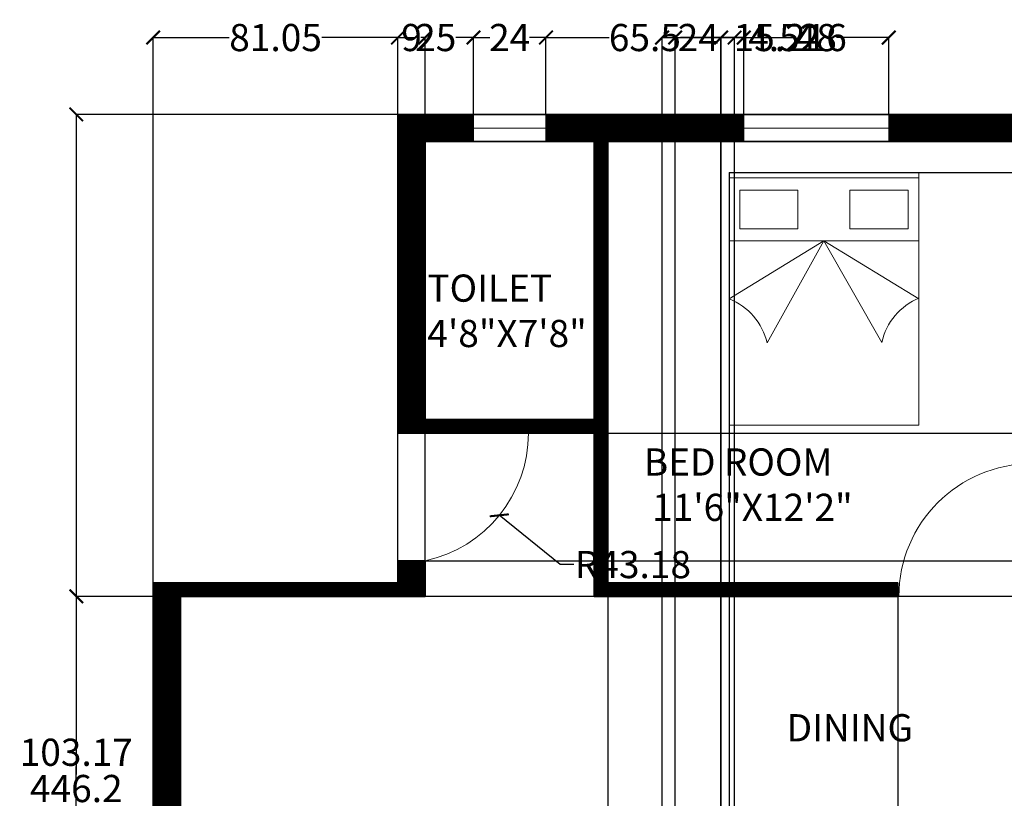
# Model space of a CAD drawing. Units: inches. Extents: x -43 to 552, y 22 to 537.
# Tile 2 of 4: x -43 to 283, y 280 to 537. Entities that reach past the tile are written whole.
import ezdxf

# ---------------------------------------------------------------- set-up
doc = ezdxf.new("R2010")
doc.units = ezdxf.units.IN
doc.header["$MEASUREMENT"] = 0
for name, color, linetype, lineweight in [('A-ANNO-DIMS', 2, 'Continuous', 18), ('A-AREA-IDEN', 7, 'Continuous', 18), ('A-DOOR', 4, 'Continuous', 18), ('A-FURN', 8, 'Continuous', 18), ('A-GLAZ', 4, 'Continuous', 18), ('A-WALL', 7, 'Continuous', 35), ('A-WALL-PATT', 252, 'Continuous', 13)]:
    doc.layers.add(name, color=color, linetype=linetype, lineweight=lineweight)
doc.styles.get("Standard").update_dxf_attribs({"font": 'arial.ttf'})
doc.dimstyles.get("Standard").update_dxf_attribs({"dimtxt": 9, "dimasz": 4.5, "dimexe": 0.18, "dimexo": 0.0625, "dimgap": 0.09, "dimtad": 0, "dimtih": 1, "dimtoh": 1, "dimdec": 1, "dimzin": 0, "dimdsep": 46, "dimlunit": 4, "dimtxsty": 'Standard', "dimblk": 'ARCHTICK', "dimcen": 0.09, "dimadec": 0, "dimazin": 0, "dimtfac": 1, "dimtdec": 1, "dimtofl": 0, "dimtmove": 0, "dimatfit": 3, "dimfxl": 1, "dimtolj": 1, "dimtzin": 0, "dimarcsym": 0})

# ---------------------------------------------------------------- blocks, each defined once
blk = doc.blocks.new('BED-DOUBLE')
for p, q in [((0, 83.65), (62.74, 83.65)), ((0, 0), (0, 83.65)), ((0, 81.91), (62.74, 81.91)), ((62.74, 83.65), (62.74, 0)), ((0, 61), (62.74, 61)), ((31.37, 61), (0, 41.83)), ((12.53, 27.23), (31.37, 61)), ((62.74, 41.83), (31.37, 61)), ((31.37, 61), (50.51, 27.4)), ((62.74, 0), (0, 0))]:
    blk.add_line(p, q)
for points in [[(3.55, 77.79), (22.76, 77.79), (22.76, 64.95), (3.55, 64.95)], [(59.19, 77.79), (39.98, 77.79), (39.98, 64.95), (59.19, 64.95)]]:
    blk.add_lwpolyline(points, close=True)
for centre, start, end in [((-7.65, 22.59), 12.9482, 68.3142), ((70.73, 22.94), 112.1918, 167.5578)]:
    blk.add_arc(centre, 20.7, start, end)
blk = doc.blocks.new('_ArchTick')
at = {"color": 0, "linetype": 'ByBlock', "const_width": 0.15}
blk.add_lwpolyline([(-0.5, -0.5), (0.5, 0.5)], dxfattribs=at)
blk = doc.blocks.new('*D9')
at = {"layer": 'A-ANNO-DIMS', "color": 0, "lineweight": -2, "transparency": 16777216}
for p, q in [((82.45, 505.95), (-24.17, 505.95)), ((-23.99, 505.95), (-23.99, 287.55)), ((-23.99, 59.77), (-23.99, 278.18)), ((289.95, 59.77), (-24.17, 59.77))]:
    blk.add_line(p, q, dxfattribs=at)
at = {"layer": 'Defpoints', "color": 0, "transparency": 16777216}
for p in [(-23.99, 505.95), (82.51, 505.95), (290.01, 59.77)]:
    blk.add_point(p, dxfattribs=at)
at = {"layer": 'A-ANNO-DIMS', "color": 0, "lineweight": -2, "transparency": 16777216, "xscale": 4.5, "yscale": 4.5, "zscale": 4.5}
for p, rotation in [((-23.99, 505.95), 90), ((-23.99, 59.77), 270)]:
    blk.add_blockref('_ArchTick', p, dxfattribs=dict(at, rotation=rotation))
at = {"layer": 'A-ANNO-DIMS', "color": 0, "transparency": 16777216, "insert": (-23.99, 282.86), "char_height": 9, "attachment_point": 5}
blk.add_mtext('\\A1;446.2', dxfattribs=at)
blk = doc.blocks.new('*D10')
at = {"layer": 'A-ANNO-DIMS', "color": 0, "lineweight": -2, "transparency": 16777216}
for p, q in [((1.46, 351.01), (1.46, 531.58)), ((1.46, 531.4), (26.67, 531.4)), ((82.51, 531.4), (57.3, 531.4)), ((82.51, 506.01), (82.51, 531.58))]:
    blk.add_line(p, q, dxfattribs=at)
at = {"layer": 'Defpoints', "color": 0, "transparency": 16777216}
for p in [(82.51, 531.4), (82.51, 505.95), (1.46, 350.95)]:
    blk.add_point(p, dxfattribs=at)
at = {"layer": 'A-ANNO-DIMS', "color": 0, "lineweight": -2, "transparency": 16777216, "xscale": 4.5, "yscale": 4.5, "zscale": 4.5, "rotation": 180}
blk.add_blockref('_ArchTick', (1.46, 531.4), dxfattribs=at)
at = {"layer": 'A-ANNO-DIMS', "color": 0, "lineweight": -2, "transparency": 16777216, "xscale": 4.5, "yscale": 4.5, "zscale": 4.5}
blk.add_blockref('_ArchTick', (82.51, 531.4), dxfattribs=at)
at = {"layer": 'A-ANNO-DIMS', "color": 0, "transparency": 16777216, "insert": (41.99, 531.4), "char_height": 9, "attachment_point": 5}
blk.add_mtext('\\A1;81.05', dxfattribs=at)
blk = doc.blocks.new('*D11')
at = {"layer": 'A-ANNO-DIMS', "color": 0, "lineweight": -2, "transparency": 16777216}
for p, q in [((82.51, 506.01), (82.51, 531.58)), ((82.51, 531.4), (88.36, 531.4)), ((107.51, 531.4), (101.66, 531.4)), ((107.51, 506.01), (107.51, 531.58))]:
    blk.add_line(p, q, dxfattribs=at)
at = {"layer": 'Defpoints', "color": 0, "transparency": 16777216}
for p in [(107.51, 531.4), (82.51, 505.95), (107.51, 505.95)]:
    blk.add_point(p, dxfattribs=at)
at = {"layer": 'A-ANNO-DIMS', "color": 0, "lineweight": -2, "transparency": 16777216, "xscale": 4.5, "yscale": 4.5, "zscale": 4.5, "rotation": 180}
blk.add_blockref('_ArchTick', (82.51, 531.4), dxfattribs=at)
at = {"layer": 'A-ANNO-DIMS', "color": 0, "lineweight": -2, "transparency": 16777216, "xscale": 4.5, "yscale": 4.5, "zscale": 4.5}
blk.add_blockref('_ArchTick', (107.51, 531.4), dxfattribs=at)
at = {"layer": 'A-ANNO-DIMS', "color": 0, "transparency": 16777216, "insert": (95.01, 531.4), "char_height": 9, "attachment_point": 5}
blk.add_mtext('\\A1;25', dxfattribs=at)
blk = doc.blocks.new('*D12')
at = {"layer": 'A-ANNO-DIMS', "color": 0, "lineweight": -2, "transparency": 16777216}
for p, q in [((107.51, 506.01), (107.51, 531.58)), ((107.51, 531.4), (112.92, 531.4)), ((131.51, 531.4), (126.11, 531.4)), ((131.51, 506.01), (131.51, 531.58))]:
    blk.add_line(p, q, dxfattribs=at)
at = {"layer": 'Defpoints', "color": 0, "transparency": 16777216}
for p in [(131.51, 531.4), (107.51, 505.95), (131.51, 505.95)]:
    blk.add_point(p, dxfattribs=at)
at = {"layer": 'A-ANNO-DIMS', "color": 0, "lineweight": -2, "transparency": 16777216, "xscale": 4.5, "yscale": 4.5, "zscale": 4.5, "rotation": 180}
blk.add_blockref('_ArchTick', (107.51, 531.4), dxfattribs=at)
at = {"layer": 'A-ANNO-DIMS', "color": 0, "lineweight": -2, "transparency": 16777216, "xscale": 4.5, "yscale": 4.5, "zscale": 4.5}
blk.add_blockref('_ArchTick', (131.51, 531.4), dxfattribs=at)
at = {"layer": 'A-ANNO-DIMS', "color": 0, "transparency": 16777216, "insert": (119.51, 531.4), "char_height": 9, "attachment_point": 5}
blk.add_mtext('\\A1;24', dxfattribs=at)
blk = doc.blocks.new('*D13')
at = {"layer": 'A-ANNO-DIMS', "color": 0, "lineweight": -2, "transparency": 16777216}
for p, q in [((131.51, 506.01), (131.51, 531.58)), ((131.51, 531.4), (152.42, 531.4)), ((197.01, 531.4), (176.1, 531.4)), ((197.01, 506.01), (197.01, 531.58))]:
    blk.add_line(p, q, dxfattribs=at)
at = {"layer": 'Defpoints', "color": 0, "transparency": 16777216}
for p in [(197.01, 531.4), (131.51, 505.95), (197.01, 505.95)]:
    blk.add_point(p, dxfattribs=at)
at = {"layer": 'A-ANNO-DIMS', "color": 0, "lineweight": -2, "transparency": 16777216, "xscale": 4.5, "yscale": 4.5, "zscale": 4.5, "rotation": 180}
blk.add_blockref('_ArchTick', (131.51, 531.4), dxfattribs=at)
at = {"layer": 'A-ANNO-DIMS', "color": 0, "lineweight": -2, "transparency": 16777216, "xscale": 4.5, "yscale": 4.5, "zscale": 4.5}
blk.add_blockref('_ArchTick', (197.01, 531.4), dxfattribs=at)
at = {"layer": 'A-ANNO-DIMS', "color": 0, "transparency": 16777216, "insert": (164.26, 531.4), "char_height": 9, "attachment_point": 5}
blk.add_mtext('\\A1;65.5', dxfattribs=at)
blk = doc.blocks.new('*D14')
at = {"layer": 'A-ANNO-DIMS', "color": 0, "lineweight": -2, "transparency": 16777216}
for p, q in [((197.01, 506.01), (197.01, 531.58)), ((197.01, 531.4), (214.28, 531.4)), ((245.01, 531.4), (227.74, 531.4)), ((245.01, 506.01), (245.01, 531.58))]:
    blk.add_line(p, q, dxfattribs=at)
at = {"layer": 'Defpoints', "color": 0, "transparency": 16777216}
for p in [(245.01, 531.4), (197.01, 505.95), (245.01, 505.95)]:
    blk.add_point(p, dxfattribs=at)
at = {"layer": 'A-ANNO-DIMS', "color": 0, "lineweight": -2, "transparency": 16777216, "xscale": 4.5, "yscale": 4.5, "zscale": 4.5, "rotation": 180}
blk.add_blockref('_ArchTick', (197.01, 531.4), dxfattribs=at)
at = {"layer": 'A-ANNO-DIMS', "color": 0, "lineweight": -2, "transparency": 16777216, "xscale": 4.5, "yscale": 4.5, "zscale": 4.5}
blk.add_blockref('_ArchTick', (245.01, 531.4), dxfattribs=at)
at = {"layer": 'A-ANNO-DIMS', "color": 0, "transparency": 16777216, "insert": (221.01, 531.4), "char_height": 9, "attachment_point": 5}
blk.add_mtext('\\A1;48', dxfattribs=at)
blk = doc.blocks.new('*D29')
at = {"layer": 'A-ANNO-DIMS', "color": 0, "lineweight": -2, "transparency": 16777216}
for p, q in [((364.95, 346.45), (-24.17, 346.45)), ((-23.99, 346.45), (-23.99, 299.55)), ((-23.99, 243.27), (-23.99, 290.17)), ((364.95, 243.27), (-24.17, 243.27))]:
    blk.add_line(p, q, dxfattribs=at)
at = {"layer": 'Defpoints', "color": 0, "transparency": 16777216}
for p in [(-23.99, 346.45), (365.01, 346.45), (365.01, 243.27)]:
    blk.add_point(p, dxfattribs=at)
at = {"layer": 'A-ANNO-DIMS', "color": 0, "lineweight": -2, "transparency": 16777216, "xscale": 4.5, "yscale": 4.5, "zscale": 4.5}
for p, rotation in [((-23.99, 346.45), 90), ((-23.99, 243.27), 270)]:
    blk.add_blockref('_ArchTick', p, dxfattribs=dict(at, rotation=rotation))
at = {"layer": 'A-ANNO-DIMS', "color": 0, "transparency": 16777216, "insert": (-23.99, 294.86), "char_height": 9, "attachment_point": 5}
blk.add_mtext('\\A1;103.17', dxfattribs=at)
blk = doc.blocks.new('*D31')
at = {"layer": 'A-ANNO-DIMS', "color": 0, "lineweight": -2, "transparency": 16777216}
for p, q in [((82.51, 358.28), (82.51, 531.58)), ((82.51, 531.4), (83.96, 531.4)), ((91.51, 531.4), (90.06, 531.4)), ((91.51, 358.28), (91.51, 531.58))]:
    blk.add_line(p, q, dxfattribs=at)
at = {"layer": 'Defpoints', "color": 0, "transparency": 16777216}
for p in [(91.51, 531.4), (82.51, 358.22), (91.51, 358.22)]:
    blk.add_point(p, dxfattribs=at)
at = {"layer": 'A-ANNO-DIMS', "color": 0, "lineweight": -2, "transparency": 16777216, "xscale": 4.5, "yscale": 4.5, "zscale": 4.5, "rotation": 180}
blk.add_blockref('_ArchTick', (82.51, 531.4), dxfattribs=at)
at = {"layer": 'A-ANNO-DIMS', "color": 0, "lineweight": -2, "transparency": 16777216, "xscale": 4.5, "yscale": 4.5, "zscale": 4.5}
blk.add_blockref('_ArchTick', (91.51, 531.4), dxfattribs=at)
at = {"layer": 'A-ANNO-DIMS', "color": 0, "transparency": 16777216, "insert": (87.01, 531.4), "char_height": 9, "attachment_point": 5}
blk.add_mtext('\\A1;9', dxfattribs=at)
blk = doc.blocks.new('*D36')
at = {"layer": 'A-ANNO-DIMS', "color": 0, "lineweight": -2, "transparency": 16777216}
for p, q in [((82.57, 400.45), (533.19, 400.45)), ((533.01, 400.45), (533.01, 384.02)), ((533.01, 358.22), (533.01, 374.64)), ((82.57, 358.22), (533.19, 358.22))]:
    blk.add_line(p, q, dxfattribs=at)
at = {"layer": 'Defpoints', "color": 0, "transparency": 16777216}
for p in [(82.51, 400.45), (533.01, 400.45), (82.51, 358.22)]:
    blk.add_point(p, dxfattribs=at)
at = {"layer": 'A-ANNO-DIMS', "color": 0, "lineweight": -2, "transparency": 16777216, "xscale": 4.5, "yscale": 4.5, "zscale": 4.5}
for p, rotation in [((533.01, 400.45), 90), ((533.01, 358.22), 270)]:
    blk.add_blockref('_ArchTick', p, dxfattribs=dict(at, rotation=rotation))
at = {"layer": 'A-ANNO-DIMS', "color": 0, "transparency": 16777216, "insert": (533.01, 379.33), "char_height": 9, "attachment_point": 5}
blk.add_mtext('\\A1;42.23', dxfattribs=at)
blk = doc.blocks.new('*D37')
at = {"layer": 'A-ANNO-DIMS', "color": 0, "lineweight": -2, "transparency": 16777216}
for p, q in [((248.01, 346.38), (248.01, 34.14)), ((290.01, 346.38), (290.01, 34.14)), ((248.01, 34.32), (262.34, 34.32)), ((290.01, 34.32), (275.68, 34.32))]:
    blk.add_line(p, q, dxfattribs=at)
at = {"layer": 'Defpoints', "color": 0, "transparency": 16777216}
for p in [(248.01, 346.45), (290.01, 346.45), (290.01, 34.32)]:
    blk.add_point(p, dxfattribs=at)
at = {"layer": 'A-ANNO-DIMS', "color": 0, "lineweight": -2, "transparency": 16777216, "xscale": 4.5, "yscale": 4.5, "zscale": 4.5, "rotation": 180}
blk.add_blockref('_ArchTick', (248.01, 34.32), dxfattribs=at)
at = {"layer": 'A-ANNO-DIMS', "color": 0, "lineweight": -2, "transparency": 16777216, "xscale": 4.5, "yscale": 4.5, "zscale": 4.5}
blk.add_blockref('_ArchTick', (290.01, 34.32), dxfattribs=at)
at = {"layer": 'A-ANNO-DIMS', "color": 0, "transparency": 16777216, "insert": (269.01, 34.32), "char_height": 9, "attachment_point": 5}
blk.add_mtext('\\A1;42', dxfattribs=at)
blk = doc.blocks.new('*D39')
at = {"layer": 'A-ANNO-DIMS', "color": 0, "lineweight": -2, "transparency": 16777216}
for p, q in [((152.01, 496.88), (152.01, 34.14)), ((192.19, 486.68), (192.19, 34.14)), ((152.01, 34.32), (156.63, 34.32)), ((192.19, 34.32), (187.56, 34.32))]:
    blk.add_line(p, q, dxfattribs=at)
at = {"layer": 'Defpoints', "color": 0, "transparency": 16777216}
for p in [(152.01, 496.95), (192.19, 486.74), (192.19, 34.32)]:
    blk.add_point(p, dxfattribs=at)
at = {"layer": 'A-ANNO-DIMS', "color": 0, "lineweight": -2, "transparency": 16777216, "xscale": 4.5, "yscale": 4.5, "zscale": 4.5, "rotation": 180}
blk.add_blockref('_ArchTick', (152.01, 34.32), dxfattribs=at)
at = {"layer": 'A-ANNO-DIMS', "color": 0, "lineweight": -2, "transparency": 16777216, "xscale": 4.5, "yscale": 4.5, "zscale": 4.5}
blk.add_blockref('_ArchTick', (192.19, 34.32), dxfattribs=at)
at = {"layer": 'A-ANNO-DIMS', "color": 0, "transparency": 16777216, "insert": (172.1, 34.32), "char_height": 9, "attachment_point": 5}
blk.add_mtext('\\A1;40.18', dxfattribs=at)
blk = doc.blocks.new('*D40')
at = {"layer": 'A-ANNO-DIMS', "color": 0, "lineweight": -2, "transparency": 16777216}
for p, q in [((197.07, 496.95), (533.19, 496.95)), ((533.01, 496.95), (533.01, 496.53)), ((192.25, 486.74), (533.19, 486.74)), ((533.01, 486.74), (533.01, 487.16))]:
    blk.add_line(p, q, dxfattribs=at)
at = {"layer": 'Defpoints', "color": 0, "transparency": 16777216}
for p in [(197.01, 496.95), (533.01, 496.95), (192.19, 486.74)]:
    blk.add_point(p, dxfattribs=at)
at = {"layer": 'A-ANNO-DIMS', "color": 0, "lineweight": -2, "transparency": 16777216, "xscale": 4.5, "yscale": 4.5, "zscale": 4.5}
for p, rotation in [((533.01, 496.95), 90), ((533.01, 486.74), 270)]:
    blk.add_blockref('_ArchTick', p, dxfattribs=dict(at, rotation=rotation))
at = {"layer": 'A-ANNO-DIMS', "color": 0, "transparency": 16777216, "insert": (533.01, 491.84), "char_height": 9, "attachment_point": 5}
blk.add_mtext('\\A1;10.204', dxfattribs=at)
blk = doc.blocks.new('*D44')
at = {"layer": 'A-ANNO-DIMS', "color": 0, "lineweight": -2, "transparency": 16777216}
for p, q in [((169.96, 255.18), (169.96, 531.58)), ((169.96, 531.4), (175.37, 531.4)), ((193.96, 531.4), (188.56, 531.4)), ((193.96, 255.18), (193.96, 531.58))]:
    blk.add_line(p, q, dxfattribs=at)
at = {"layer": 'Defpoints', "color": 0, "transparency": 16777216}
for p in [(193.96, 531.4), (169.96, 255.12), (193.96, 255.12)]:
    blk.add_point(p, dxfattribs=at)
at = {"layer": 'A-ANNO-DIMS', "color": 0, "lineweight": -2, "transparency": 16777216, "xscale": 4.5, "yscale": 4.5, "zscale": 4.5, "rotation": 180}
blk.add_blockref('_ArchTick', (169.96, 531.4), dxfattribs=at)
at = {"layer": 'A-ANNO-DIMS', "color": 0, "lineweight": -2, "transparency": 16777216, "xscale": 4.5, "yscale": 4.5, "zscale": 4.5}
blk.add_blockref('_ArchTick', (193.96, 531.4), dxfattribs=at)
at = {"layer": 'A-ANNO-DIMS', "color": 0, "transparency": 16777216, "insert": (181.96, 531.4), "char_height": 9, "attachment_point": 5}
blk.add_mtext('\\A1;24', dxfattribs=at)
blk = doc.blocks.new('*D49')
at = {"layer": 'A-ANNO-DIMS', "color": 0, "lineweight": -2, "transparency": 16777216}
for p, q in [((174.31, 245.11), (174.31, 531.58)), ((174.31, 531.4), (189.53, 531.4)), ((189.53, 245.11), (189.53, 531.58)), ((189.53, 531.4), (194.03, 531.4))]:
    blk.add_line(p, q, dxfattribs=at)
at = {"layer": 'Defpoints', "color": 0, "transparency": 16777216}
for p in [(189.53, 531.4), (174.31, 245.05), (189.53, 245.05)]:
    blk.add_point(p, dxfattribs=at)
at = {"layer": 'A-ANNO-DIMS', "color": 0, "lineweight": -2, "transparency": 16777216, "xscale": 4.5, "yscale": 4.5, "zscale": 4.5, "rotation": 180}
blk.add_blockref('_ArchTick', (174.31, 531.4), dxfattribs=at)
at = {"layer": 'A-ANNO-DIMS', "color": 0, "lineweight": -2, "transparency": 16777216, "xscale": 4.5, "yscale": 4.5, "zscale": 4.5}
blk.add_blockref('_ArchTick', (189.53, 531.4), dxfattribs=at)
at = {"layer": 'A-ANNO-DIMS', "color": 0, "transparency": 16777216, "insert": (212.37, 531.4), "char_height": 9, "attachment_point": 5}
blk.add_mtext('\\A1;15.216', dxfattribs=at)
blk = doc.blocks.new('*D53')
at = {"layer": 'A-ANNO-DIMS', "color": 0, "lineweight": -2, "transparency": 16777216}
for p, q in [((189.45, 165.34), (189.45, 531.58)), ((189.45, 531.4), (193.96, 531.4)), ((193.96, 146.51), (193.96, 531.58)), ((193.96, 531.4), (198.46, 531.4))]:
    blk.add_line(p, q, dxfattribs=at)
at = {"layer": 'Defpoints', "color": 0, "transparency": 16777216}
for p in [(193.96, 531.4), (189.45, 165.27), (193.96, 146.45)]:
    blk.add_point(p, dxfattribs=at)
at = {"layer": 'A-ANNO-DIMS', "color": 0, "lineweight": -2, "transparency": 16777216, "xscale": 4.5, "yscale": 4.5, "zscale": 4.5, "rotation": 180}
blk.add_blockref('_ArchTick', (189.45, 531.4), dxfattribs=at)
at = {"layer": 'A-ANNO-DIMS', "color": 0, "lineweight": -2, "transparency": 16777216, "xscale": 4.5, "yscale": 4.5, "zscale": 4.5}
blk.add_blockref('_ArchTick', (193.96, 531.4), dxfattribs=at)
at = {"layer": 'A-ANNO-DIMS', "color": 0, "transparency": 16777216, "insert": (210.38, 531.4), "char_height": 9, "attachment_point": 5}
blk.add_mtext('\\A1;4.52', dxfattribs=at)
blk = doc.blocks.new('*D56')
at = {"layer": 'A-ANNO-DIMS', "color": 0, "lineweight": -2, "transparency": 16777216}
for p, q in [((82.42, 400.45), (82.6, 400.45)), ((82.51, 400.36), (82.51, 400.54)), ((136.21, 356.98), (116.07, 373.28)), ((140.71, 356.98), (136.21, 356.98))]:
    blk.add_line(p, q, dxfattribs=at)
at = {"layer": 'Defpoints', "color": 0, "transparency": 16777216}
for p in [(82.51, 400.45), (116.07, 373.28)]:
    blk.add_point(p, dxfattribs=at)
at = {"layer": 'A-ANNO-DIMS', "color": 0, "lineweight": -2, "transparency": 16777216, "xscale": 4.5, "yscale": 4.5, "zscale": 4.5, "rotation": 141.0154171181597}
blk.add_blockref('_ArchTick', (116.07, 373.28), dxfattribs=at)
at = {"layer": 'A-ANNO-DIMS', "color": 0, "transparency": 16777216, "insert": (160.3, 356.98), "char_height": 9, "attachment_point": 5}
blk.add_mtext('\\A1;R43.18', dxfattribs=at)

msp = doc.modelspace()

# ---------------------------------------------------------------- hatches: boundary and pattern name
at = {"layer": 'A-WALL-PATT'}
h = msp.add_hatch(dxfattribs=at)
h.set_pattern_fill('ANSI31', color=256)
h.set_pattern_definition([(45, (-523.11303, 0), (-0.088388348, 0.088388348), [])])
h.paths.add_polyline_path([(202.9985, 146.4471), (169.965, 146.4471), (169.965, 255.1157), (165.465, 255.1157), (165.465, 146.4471), (147.9805, 146.4471), (147.9805, 141.9471), (165.465, 141.9471), (165.465, 84.9471), (169.965, 84.9471), (169.965, 141.9471), (202.9985, 141.9471)])
h.paths.add_polyline_path([(294.5106, 146.4471), (294.5106, 238.775), (294.5106, 243.275), (294.5106, 255.1157), (290.0106, 255.1157), (290.0106, 146.4471), (247.8411, 146.4471), (247.8411, 141.9471), (290.0106, 141.9471), (290.0106, 93.9471), (290.0106, 59.775), (294.5106, 59.775), (294.5106, 77.3814), (294.5106, 93.9471), (294.5106, 107.775), (316.2676, 107.775), (316.2676, 116.775), (294.5106, 116.775)])
h.paths.add_polyline_path([(10.465, 346.4471), (82.5106, 346.4471), (91.5106, 346.4471), (91.5106, 358.2163), (82.5106, 358.2163), (82.5106, 350.9471), (1.465, 350.9471), (1.465, 84.9471), (10.465, 84.9471), (10.465, 141.9471), (56.4237, 141.9471), (56.4237, 146.4471), (10.465, 146.4471)])
h.paths.add_polyline_path([(91.5106, 496.9471), (107.5106, 496.9471), (107.5106, 505.9471), (82.5106, 505.9471), (82.5106, 400.4471), (147.5106, 400.4471), (147.5106, 346.4471), (248.0106, 346.4471), (248.0106, 350.9471), (152.0106, 350.9471), (152.0106, 496.9471), (197.0106, 496.9471), (197.0106, 505.9471), (131.5106, 505.9471), (131.5106, 496.9471), (147.5106, 496.9471), (147.5106, 404.9471), (91.5106, 404.9471)])
h.paths.add_polyline_path([(477.5106, 505.9471), (245.0106, 505.9471), (245.0106, 496.9471), (290.0106, 496.9471), (290.0106, 390.2693, -0.02565505), (294.5106, 390.2693), (294.5106, 496.9471), (468.5106, 496.9471), (468.5106, 460.1763), (477.5106, 460.1763)])

# ---------------------------------------------------------------- linework, layer by layer
at = {"layer": 'A-DOOR'}
for p, q in [((82.5106, 400.4471), (82.5106, 358.2163)), ((290.0106, 346.4471), (248.0106, 346.4471)), ((248.0106, 346.4471), (294.5106, 346.4471))]:
    msp.add_line(p, q, dxfattribs=at)
for centre, radius, start, end in [((82.5106, 400.4471), 43.1792, 282.030572, 0), ((292.2606, 346.4471), 43.8799, 0, 180)]:
    msp.add_arc(centre, radius, start, end, dxfattribs=at)
at = {"layer": 'A-GLAZ'}
for p, q in [((107.5106, 496.9471), (107.5106, 505.9471)), ((131.5106, 496.9471), (131.5106, 505.9471)), ((197.0106, 496.9471), (197.0106, 505.9471)), ((245.0106, 496.9471), (245.0106, 505.9471)), ((107.5106, 501.4471), (131.5106, 501.4471)), ((197.0106, 501.4471), (245.0106, 501.4471))]:
    msp.add_line(p, q, dxfattribs=at)
at = {"layer": 'A-WALL'}
for p, q in [((82.5106, 505.9471), (477.5106, 505.9471)), ((82.5106, 505.9471), (82.5106, 400.4471)), ((91.5106, 496.9471), (147.5106, 496.9471)), ((91.5106, 496.9471), (91.5106, 404.9471)), ((147.5106, 496.9471), (147.5106, 404.9471)), ((152.0106, 496.9471), (152.0106, 350.9471)), ((152.0106, 496.9471), (290.0106, 496.9471)), ((91.5106, 404.9471), (147.5106, 404.9471)), ((82.5106, 400.4471), (147.5106, 400.4471)), ((147.5106, 400.4471), (147.5106, 346.4471)), ((82.5106, 358.2163), (91.5106, 358.2163)), ((82.5106, 358.2163), (82.5106, 350.9471)), ((91.5106, 358.2163), (91.5106, 346.4471)), ((1.465, 350.9471), (1.465, 84.9471)), ((82.5106, 350.9471), (1.465, 350.9471)), ((152.0106, 350.9471), (248.0106, 350.9471)), ((248.0106, 350.9471), (248.0106, 346.4471)), ((10.465, 346.4471), (10.465, 146.4471)), ((82.5106, 346.4471), (10.465, 346.4471)), ((82.5106, 346.4471), (91.5106, 346.4471)), ((147.5106, 346.4471), (248.0106, 346.4471))]:
    msp.add_line(p, q, dxfattribs=at)

# ---------------------------------------------------------------- block references
at = {"layer": 'A-FURN'}
msp.add_blockref('BED-DOUBLE', (192.1876, 403.0902), dxfattribs=at)

# ---------------------------------------------------------------- texts
at = {"layer": 'A-AREA-IDEN', "char_height": 9, "attachment_point": 1}
for s, insert in [('  TOILET\\P  4\'8"X7\'8"', (86.7539, 452.9656)), ('BED ROOM\\P 11\'6"X12\'2"', (163.9139, 395.4191)), ('DINING', (211.1952, 307.4695))]:
    msp.add_mtext_dynamic_manual_height_columns(s, width=549.697564, gutter_width=1, heights=[0], dxfattribs=dict(at, insert=insert))

# ---------------------------------------------------------------- dimensions: what is measured, and where the dimension line sits
at = {"layer": 'A-ANNO-DIMS'}
for base, p1, p2, override, picture, middle in [((82.5106, 531.3971), (1.465, 350.9471), (82.5106, 505.9471), {"dimdec": 2, "dimlfac": 1, "dimrnd": 0, "dimzin": 0, "dimdsep": 46, "dimlunit": 2}, '*D10', (41.9878, 531.3971)), ((107.5106, 531.3971), (82.5106, 505.9471), (107.5106, 505.9471), {"dimdec": 0, "dimlfac": 1, "dimrnd": 0, "dimzin": 0, "dimdsep": 46, "dimlunit": 2}, '*D11', (95.0106, 531.3971)), ((91.5106, 531.3971), (82.5106, 358.2163), (91.5106, 358.2163), {"dimdec": 0, "dimlfac": 1, "dimrnd": 0, "dimzin": 0, "dimdsep": 46, "dimlunit": 2}, '*D31', (87.0106, 531.3971)), ((131.5106, 531.3971), (107.5106, 505.9471), (131.5106, 505.9471), {"dimdec": 0, "dimlfac": 1, "dimrnd": 0, "dimzin": 0, "dimdsep": 46, "dimlunit": 2}, '*D12', (119.5106, 531.3971)), ((197.0106, 531.3971), (131.5106, 505.9471), (197.0106, 505.9471), {"dimdec": 1, "dimlfac": 1, "dimrnd": 0, "dimzin": 0, "dimdsep": 46, "dimlunit": 2}, '*D13', (164.2606, 531.3971)), ((193.965, 531.3971), (169.965, 255.1157), (193.965, 255.1157), {"dimdec": 0, "dimlfac": 1, "dimrnd": 0, "dimzin": 0, "dimdsep": 46, "dimlunit": 2}, '*D44', (181.965, 531.3971)), ((189.5259, 531.3971), (174.3101, 245.0503), (189.5259, 245.0503), {"dimdec": 3, "dimlfac": 1, "dimrnd": 0, "dimzin": 0, "dimdsep": 46, "dimlunit": 2}, '*D49', (212.3707, 531.3971)), ((193.965, 531.3971), (189.4495, 165.2726), (193.965, 146.4471), {"dimdec": 2, "dimlfac": 1, "dimrnd": 0, "dimzin": 0, "dimdsep": 46, "dimlunit": 2}, '*D53', (210.379, 531.3971)), ((245.0106, 531.3971), (197.0106, 505.9471), (245.0106, 505.9471), {"dimdec": 0, "dimlfac": 1, "dimrnd": 0, "dimzin": 0, "dimdsep": 46, "dimlunit": 2}, '*D14', (221.0106, 531.3971)), ((192.1876, 34.325), (152.0106, 496.9471), (192.1876, 486.7427), {"dimdec": 2, "dimlfac": 1, "dimrnd": 0, "dimzin": 0, "dimdsep": 46, "dimlunit": 2}, '*D39', (172.0991, 34.325)), ((290.0106, 34.325), (248.0106, 346.4471), (290.0106, 346.4471), {"dimdec": 0, "dimlfac": 1, "dimrnd": 0, "dimzin": 0, "dimdsep": 46, "dimlunit": 2}, '*D37', (269.0106, 34.325))]:
    dim = msp.add_linear_dim(base=base, p1=p1, p2=p2, dimstyle='Standard', override=override, dxfattribs=at)
    dim.commit()
    dim.dimension.update_dxf_attribs({"geometry": picture, "text_midpoint": middle})
for base, p1, p2, override, picture, middle in [((-23.985, 505.9471), (290.0106, 59.775), (82.5106, 505.9471), {"dimdec": 1, "dimlfac": 1, "dimrnd": 0, "dimzin": 0, "dimdsep": 46, "dimlunit": 2}, '*D9', (-23.985, 282.8611)), ((533.0111, 496.9471), (192.1876, 486.7427), (197.0106, 496.9471), {"dimdec": 3, "dimlfac": 1, "dimrnd": 0, "dimzin": 0, "dimdsep": 46, "dimlunit": 2}, '*D40', (533.0111, 491.8449)), ((533.0111, 400.4471), (82.5106, 358.2163), (82.5106, 400.4471), {"dimdec": 2, "dimlfac": 1, "dimrnd": 0, "dimzin": 0, "dimdsep": 46, "dimlunit": 2}, '*D36', (533.0111, 379.3317)), ((-23.985, 346.4471), (365.0106, 243.275), (365.0106, 346.4471), {"dimdec": 2, "dimlfac": 1, "dimrnd": 0, "dimzin": 0, "dimdsep": 46, "dimlunit": 2}, '*D29', (-23.985, 294.8611))]:
    dim = msp.add_linear_dim(base=base, p1=p1, p2=p2, angle=90, dimstyle='Standard', override=override, dxfattribs=at)
    dim.commit()
    dim.dimension.update_dxf_attribs({"geometry": picture, "text_midpoint": middle})
dim = msp.add_radius_dim(center=(82.5106, 400.4471), mpoint=(116.0745, 373.2826), dimstyle='Standard', override={"dimdec": 2, "dimlfac": 1, "dimrnd": 0, "dimzin": 0, "dimdsep": 46, "dimlunit": 2}, dxfattribs=at)
dim.commit()
dim.dimension.update_dxf_attribs({"geometry": '*D56', "text_midpoint": (160.3038, 356.9839), "dimtype": 164})

doc.saveas('drawing.dxf')
